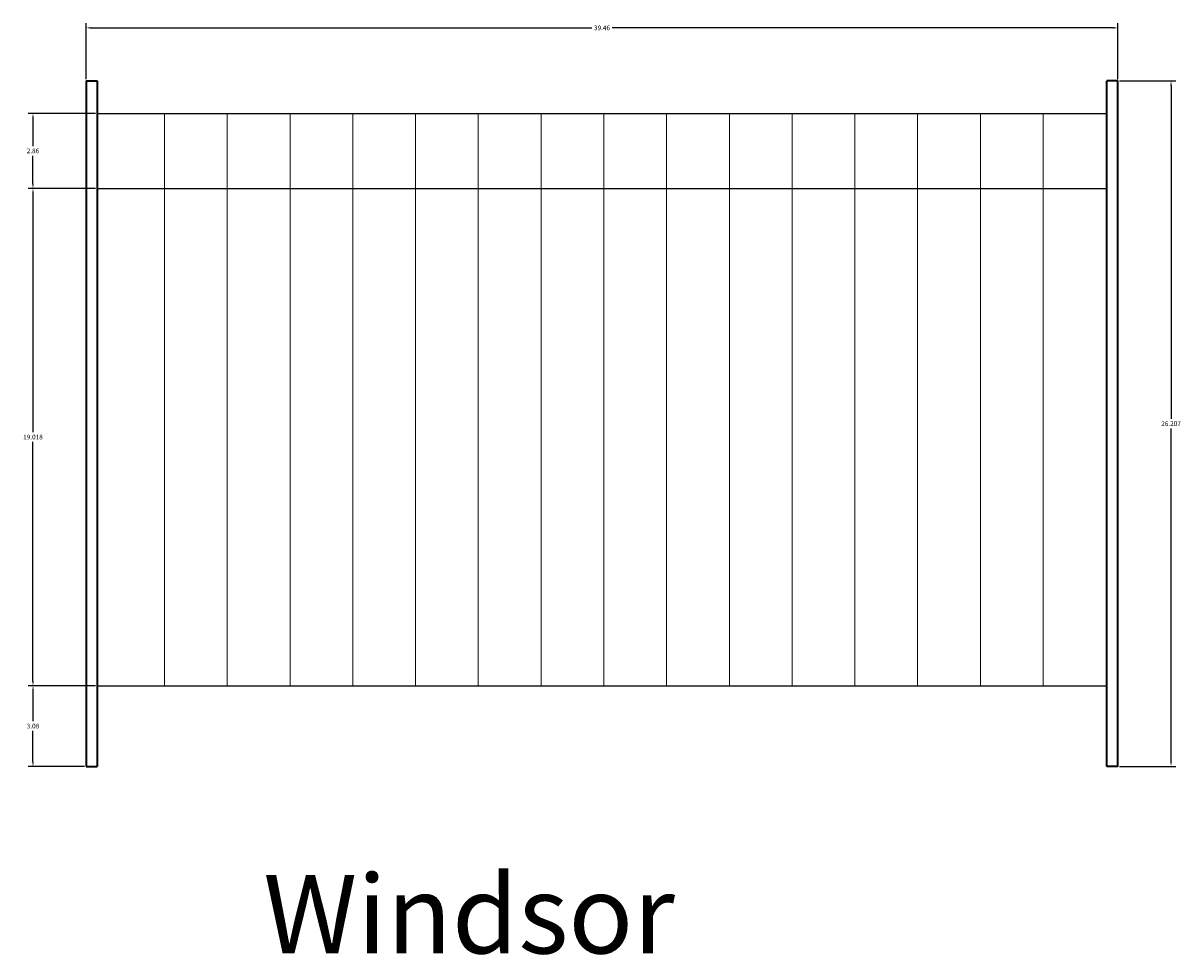
# Model space of a CAD drawing. Units: inches. Extents: x 756 to 915, y 488 to 695.
# Tile 10 of 25: x 864 to 908, y 547 to 583. Entities that reach past the tile are written whole.
import ezdxf

# ---------------------------------------------------------------- set-up
doc = ezdxf.new("R2010")
doc.units = ezdxf.units.IN
doc.header["$MEASUREMENT"] = 0
for name, color, linetype, lineweight in [('L-ANNO-TEXT', 7, 'Continuous', 25), ('L-FENC-PCKT', 7, 'Continuous', 18), ('L-FENC-POST', 7, 'Continuous', 35), ('L-FENC-RAIL', 7, 'Continuous', 25), ('M-DIMS', 2, 'Continuous', 18)]:
    doc.layers.add(name, color=color, linetype=linetype, lineweight=lineweight)
doc.styles.get("Standard").update_dxf_attribs({"font": 'arial.ttf'})
doc.dimstyles.get("Standard").update_dxf_attribs({"dimtxt": 0.18, "dimasz": 0.18, "dimexe": 0.18, "dimexo": 0.0625, "dimgap": 0.09, "dimtad": 0, "dimtih": 1, "dimtoh": 1, "dimdec": 0, "dimzin": 0, "dimdsep": 46, "dimlunit": 3, "dimtxsty": 'Standard', "dimcen": 0.09, "dimadec": 0, "dimazin": 0, "dimtfac": 1, "dimtdec": 0, "dimtofl": 0, "dimtmove": 0, "dimatfit": 3, "dimfxl": 1, "dimtolj": 1, "dimtzin": 0, "dimarcsym": 0})

# ---------------------------------------------------------------- blocks, each defined once
blk = doc.blocks.new('FENCE-POST-LEFT')
for p, q in [((0, 26.207), (0, 0)), ((0, 26.207), (0.426, 26.207)), ((0.426, 26.207), (0.426, 0)), ((0.426, 26.207), (0.426, 0)), ((0, 0), (0.426, 0))]:
    blk.add_line(p, q)
blk = doc.blocks.new('FENCE-POST-RIGHT')
for p, q in [((0, 26.207), (0, 0)), ((0, 26.207), (0.427, 26.207)), ((0.427, 26.207), (0.427, 0)), ((0, 0), (0.427, 0))]:
    blk.add_line(p, q)
blk = doc.blocks.new('*D58')
at = {"layer": 'Defpoints', "color": 0, "transparency": 16777216}
for p in [(905.684, 582.577), (866.226, 580.547), (905.684, 580.547)]:
    blk.add_point(p, dxfattribs=at)
at = {"layer": 'M-DIMS', "color": 0, "lineweight": -2, "transparency": 16777216}
for p, q in [((866.226, 580.61), (866.226, 582.757)), ((866.406, 582.577), (885.561, 582.577)), ((905.504, 582.577), (886.348, 582.577)), ((905.684, 580.61), (905.684, 582.757))]:
    blk.add_line(p, q, dxfattribs=at)
at = {"layer": 'M-DIMS', "color": 0, "transparency": 16777216}
for points in [[(866.406, 582.607), (866.406, 582.547), (866.226, 582.577)], [(905.504, 582.607), (905.504, 582.547), (905.684, 582.577)]]:
    blk.add_solid(points, dxfattribs=at)
at = {"layer": 'M-DIMS', "color": 0, "transparency": 16777216, "insert": (885.955, 582.577), "char_height": 0.18, "attachment_point": 5}
blk.add_mtext('\\A1;39.46', dxfattribs=at)
blk = doc.blocks.new('*D59')
at = {"layer": 'Defpoints', "color": 0, "transparency": 16777216}
for p in [(905.684, 580.547), (907.714, 580.547), (905.684, 554.34)]:
    blk.add_point(p, dxfattribs=at)
at = {"layer": 'M-DIMS', "color": 0, "lineweight": -2, "transparency": 16777216}
for p, q in [((905.746, 580.547), (907.894, 580.547)), ((907.714, 580.367), (907.714, 567.626)), ((907.714, 554.52), (907.714, 567.262)), ((905.746, 554.34), (907.894, 554.34))]:
    blk.add_line(p, q, dxfattribs=at)
at = {"layer": 'M-DIMS', "color": 0, "transparency": 16777216}
for points in [[(907.684, 580.367), (907.744, 580.367), (907.714, 580.547)], [(907.684, 554.52), (907.744, 554.52), (907.714, 554.34)]]:
    blk.add_solid(points, dxfattribs=at)
at = {"layer": 'M-DIMS', "color": 0, "transparency": 16777216, "insert": (907.714, 567.444), "char_height": 0.18, "attachment_point": 5}
blk.add_mtext('\\A1;26.207', dxfattribs=at)
blk = doc.blocks.new('*D60')
at = {"layer": 'Defpoints', "color": 0, "transparency": 16777216}
for p in [(864.196, 557.422), (866.652, 557.422), (866.226, 554.34)]:
    blk.add_point(p, dxfattribs=at)
at = {"layer": 'M-DIMS', "color": 0, "lineweight": -2, "transparency": 16777216}
for p, q in [((866.59, 557.422), (864.016, 557.422)), ((864.196, 557.242), (864.196, 556.063)), ((864.196, 554.52), (864.196, 555.699)), ((866.163, 554.34), (864.016, 554.34))]:
    blk.add_line(p, q, dxfattribs=at)
at = {"layer": 'M-DIMS', "color": 0, "transparency": 16777216}
for points in [[(864.166, 557.242), (864.226, 557.242), (864.196, 557.422)], [(864.166, 554.52), (864.226, 554.52), (864.196, 554.34)]]:
    blk.add_solid(points, dxfattribs=at)
at = {"layer": 'M-DIMS', "color": 0, "transparency": 16777216, "insert": (864.196, 555.881), "char_height": 0.18, "attachment_point": 5}
blk.add_mtext('\\A1;3.08', dxfattribs=at)
blk = doc.blocks.new('*D61')
at = {"layer": 'Defpoints', "color": 0, "transparency": 16777216}
for p in [(864.196, 576.44), (866.652, 576.44), (866.652, 557.422)]:
    blk.add_point(p, dxfattribs=at)
at = {"layer": 'M-DIMS', "color": 0, "lineweight": -2, "transparency": 16777216}
for p, q in [((866.59, 576.44), (864.016, 576.44)), ((864.196, 576.26), (864.196, 567.113)), ((864.196, 557.602), (864.196, 566.749)), ((866.59, 557.422), (864.016, 557.422))]:
    blk.add_line(p, q, dxfattribs=at)
at = {"layer": 'M-DIMS', "color": 0, "transparency": 16777216}
for points in [[(864.166, 576.26), (864.226, 576.26), (864.196, 576.44)], [(864.166, 557.602), (864.226, 557.602), (864.196, 557.422)]]:
    blk.add_solid(points, dxfattribs=at)
at = {"layer": 'M-DIMS', "color": 0, "transparency": 16777216, "insert": (864.196, 566.931), "char_height": 0.18, "attachment_point": 5}
blk.add_mtext('\\A1;19.018', dxfattribs=at)
blk = doc.blocks.new('*D62')
at = {"layer": 'Defpoints', "color": 0, "transparency": 16777216}
for p in [(864.196, 579.304), (866.652, 579.304), (866.652, 576.44)]:
    blk.add_point(p, dxfattribs=at)
at = {"layer": 'M-DIMS', "color": 0, "lineweight": -2, "transparency": 16777216}
for p, q in [((866.59, 579.304), (864.016, 579.304)), ((864.196, 579.124), (864.196, 578.054)), ((864.196, 576.62), (864.196, 577.69)), ((866.59, 576.44), (864.016, 576.44))]:
    blk.add_line(p, q, dxfattribs=at)
at = {"layer": 'M-DIMS', "color": 0, "transparency": 16777216}
for points in [[(864.166, 579.124), (864.226, 579.124), (864.196, 579.304)], [(864.166, 576.62), (864.226, 576.62), (864.196, 576.44)]]:
    blk.add_solid(points, dxfattribs=at)
at = {"layer": 'M-DIMS', "color": 0, "transparency": 16777216, "insert": (864.196, 577.872), "char_height": 0.18, "attachment_point": 5}
blk.add_mtext('\\A1;2.86', dxfattribs=at)

msp = doc.modelspace()

# ---------------------------------------------------------------- linework, layer by layer
at = {"layer": 'L-FENC-PCKT'}
for p, q in [((869.2247, 579.3043), (869.2247, 557.422)), ((871.6246, 579.3043), (871.6246, 557.422)), ((874.0245, 579.3043), (874.0245, 557.422)), ((876.4244, 579.3043), (876.4244, 557.422)), ((878.8243, 579.3043), (878.8243, 557.422)), ((881.2242, 579.3043), (881.2242, 557.422)), ((883.6241, 579.3043), (883.6241, 557.422)), ((886.024, 579.3043), (886.024, 557.422)), ((888.4239, 579.3043), (888.4239, 557.422)), ((890.8239, 579.3043), (890.8239, 557.422)), ((893.2238, 579.3043), (893.2238, 557.422)), ((895.6237, 579.3043), (895.6237, 557.422)), ((898.0236, 579.3043), (898.0236, 557.422)), ((900.4235, 579.3043), (900.4235, 557.422)), ((902.8234, 579.3043), (902.8234, 557.422))]:
    msp.add_line(p, q, dxfattribs=at)
at = {"layer": 'L-FENC-RAIL'}
for p, q in [((866.6522, 579.3043), (905.257, 579.3043)), ((866.6522, 576.4399), (905.257, 576.4399)), ((866.6522, 557.422), (905.257, 557.422))]:
    msp.add_line(p, q, dxfattribs=at)

# ---------------------------------------------------------------- block references
at = {"layer": 'L-FENC-POST'}
msp.add_blockref('FENCE-POST-LEFT', (866.2259, 554.3403), dxfattribs=at)
at = {"layer": 'L-FENC-POST', "rotation": 180}
msp.add_blockref('FENCE-POST-RIGHT', (905.6838, 580.5473), dxfattribs=at)

# ---------------------------------------------------------------- texts
at = {"layer": 'L-ANNO-TEXT'}
msp.add_text('Windsor', height=3, dxfattribs=at).set_placement((873.0013, 547.1859))

# ---------------------------------------------------------------- dimensions: what is measured, and where the dimension line sits
at = {"layer": 'M-DIMS'}
dim = msp.add_linear_dim(base=(905.6837, 582.5772), p1=(866.2255, 580.5472), p2=(905.6837, 580.5472), dimstyle='Standard', override={"dimdec": 2, "dimlfac": 1, "dimrnd": 0, "dimzin": 0, "dimdsep": 46, "dimlunit": 2}, dxfattribs=at)
dim.commit()
dim.dimension.update_dxf_attribs({"geometry": '*D58', "text_midpoint": (885.9546, 582.5772)})
for base, p1, p2, override, picture, middle in [((907.7137, 580.5472), (905.6837, 554.3404), (905.6837, 580.5472), {"dimdec": 3, "dimlfac": 1, "dimrnd": 0, "dimzin": 0, "dimdsep": 46, "dimlunit": 2}, '*D59', (907.7137, 567.4438)), ((864.1955, 579.3043), (866.6522, 576.4399), (866.6522, 579.3043), {"dimdec": 2, "dimlfac": 1, "dimrnd": 0, "dimzin": 0, "dimdsep": 46, "dimlunit": 2}, '*D62', (864.1955, 577.8721)), ((864.1955, 576.4399), (866.6522, 557.422), (866.6522, 576.4399), {"dimdec": 3, "dimlfac": 1, "dimrnd": 0, "dimzin": 0, "dimdsep": 46, "dimlunit": 2}, '*D61', (864.1955, 566.931)), ((864.1955, 557.422), (866.2255, 554.3404), (866.6522, 557.422), {"dimdec": 2, "dimlfac": 1, "dimrnd": 0, "dimzin": 0, "dimdsep": 46, "dimlunit": 2}, '*D60', (864.1955, 555.8812))]:
    dim = msp.add_linear_dim(base=base, p1=p1, p2=p2, angle=90, dimstyle='Standard', override=override, dxfattribs=at)
    dim.commit()
    dim.dimension.update_dxf_attribs({"geometry": picture, "text_midpoint": middle})

doc.saveas('drawing.dxf')
